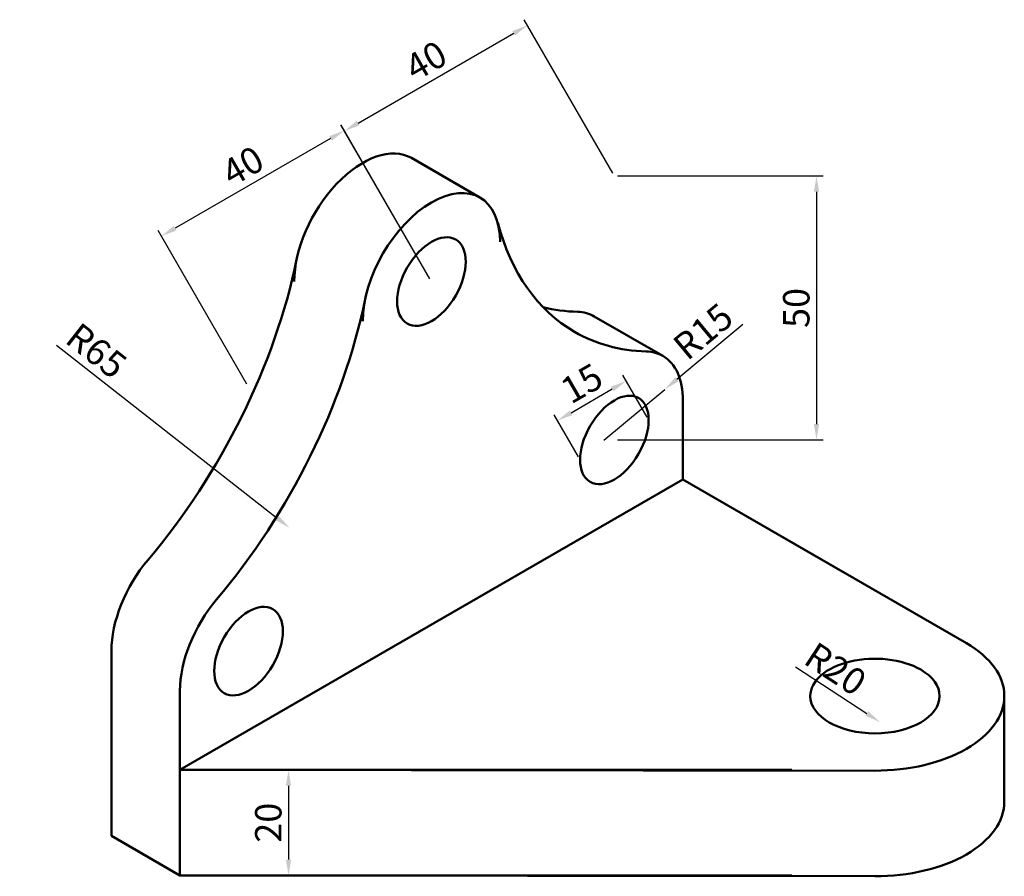
# Model space of a CAD drawing. Units: millimetres. Extents: x 6 to 193, y 3 to 166.
import ezdxf

# ---------------------------------------------------------------- set-up
doc = ezdxf.new("R2010")
doc.units = ezdxf.units.MM
doc.layers.add('M-DIMS', color=2, linetype='Continuous', lineweight=25)
doc.layers.add('M-OUTL', color=7, linetype='Continuous', lineweight=50)
doc.styles.get("Standard").update_dxf_attribs({"font": 'arial.ttf'})
doc.dimstyles.new('ISO-25', dxfattribs={"dimtxt": 5, "dimasz": 3, "dimexe": 1.25, "dimexo": 0.625, "dimtad": 1, "dimtxsty": 'Standard', "dimcen": 2.5, "dimadec": 0, "dimazin": 0, "dimtfac": 1, "dimtmove": 0, "dimatfit": 3, "dimfxl": 1, "dimarcsym": 0})

# ---------------------------------------------------------------- blocks, each defined once
blk = doc.blocks.new('*D1')
at = {"layer": 'Defpoints', "color": 0, "transparency": 16777216}
for p in [(118.67, 136.1), (118.67, 86.1), (156.96, 86.1)]:
    blk.add_point(p, dxfattribs=at)
at = {"layer": 'M-DIMS', "color": 0, "lineweight": -2, "transparency": 16777216}
for p, q in [((119.3, 136.1), (158.21, 136.1)), ((156.96, 133.1), (156.96, 89.1)), ((119.3, 86.1), (158.21, 86.1))]:
    blk.add_line(p, q, dxfattribs=at)
at = {"layer": 'M-DIMS', "color": 0, "transparency": 16777216}
for points in [[(156.46, 133.1), (157.46, 133.1), (156.96, 136.1)], [(156.46, 89.1), (157.46, 89.1), (156.96, 86.1)]]:
    blk.add_solid(points, dxfattribs=at)
at = {"layer": 'M-DIMS', "color": 0, "transparency": 16777216, "insert": (153.78, 111.1), "char_height": 5, "attachment_point": 5, "rotation": 90}
blk.add_mtext('50', dxfattribs=at)
blk = doc.blocks.new('*D2')
at = {"layer": 'Defpoints', "color": 0, "transparency": 16777216}
for p in [(102.21, 164.62), (118.67, 136.1), (84.03, 116.1)]:
    blk.add_point(p, dxfattribs=at)
at = {"layer": 'M-DIMS', "color": 0, "lineweight": -2, "transparency": 16777216}
for p, q in [((118.36, 136.64), (101.58, 165.7)), ((70.16, 146.12), (99.61, 163.12)), ((83.72, 116.64), (66.94, 145.7))]:
    blk.add_line(p, q, dxfattribs=at)
at = {"layer": 'M-DIMS', "color": 0, "transparency": 16777216}
for points in [[(99.36, 163.55), (99.86, 162.69), (102.21, 164.62)], [(69.91, 146.55), (70.41, 145.69), (67.56, 144.62)]]:
    blk.add_solid(points, dxfattribs=at)
at = {"layer": 'M-DIMS', "color": 0, "transparency": 16777216, "insert": (83.3, 157.37), "char_height": 5, "attachment_point": 5, "rotation": 30}
blk.add_mtext('40', dxfattribs=at)
blk = doc.blocks.new('*D3')
at = {"layer": 'Defpoints', "color": 0, "transparency": 16777216}
for p in [(32.88, 124.7), (84.03, 116.1), (49.39, 96.1)]:
    blk.add_point(p, dxfattribs=at)
at = {"layer": 'M-DIMS', "color": 0, "lineweight": -2, "transparency": 16777216}
for p, q in [((83.72, 116.64), (66.89, 145.78)), ((64.92, 143.2), (35.48, 126.2)), ((49.08, 96.64), (32.25, 125.78))]:
    blk.add_line(p, q, dxfattribs=at)
at = {"layer": 'M-DIMS', "color": 0, "transparency": 16777216}
for points in [[(64.67, 143.63), (65.17, 142.76), (67.52, 144.7)], [(35.23, 126.63), (35.73, 125.76), (32.88, 124.7)]]:
    blk.add_solid(points, dxfattribs=at)
at = {"layer": 'M-DIMS', "color": 0, "transparency": 16777216, "insert": (48.61, 137.45), "char_height": 5, "attachment_point": 5, "rotation": 30}
blk.add_mtext('40', dxfattribs=at)
blk = doc.blocks.new('*D4')
at = {"layer": 'Defpoints', "color": 0, "transparency": 16777216}
for p in [(36.4, 23.6), (36.4, 3.6), (56.96, 3.6)]:
    blk.add_point(p, dxfattribs=at)
at = {"layer": 'M-DIMS', "color": 0, "lineweight": -2, "transparency": 16777216}
for p, q in [((37.03, 23.6), (58.21, 23.6)), ((56.96, 20.6), (56.96, 6.6)), ((37.03, 3.6), (58.21, 3.6))]:
    blk.add_line(p, q, dxfattribs=at)
at = {"layer": 'M-DIMS', "color": 0, "transparency": 16777216}
for points in [[(56.46, 20.6), (57.46, 20.6), (56.96, 23.6)], [(56.46, 6.6), (57.46, 6.6), (56.96, 3.6)]]:
    blk.add_solid(points, dxfattribs=at)
at = {"layer": 'M-DIMS', "color": 0, "transparency": 16777216, "insert": (53.78, 13.6), "char_height": 5, "attachment_point": 5, "rotation": 90}
blk.add_mtext('20', dxfattribs=at)
blk = doc.blocks.new('*D5')
at = {"layer": 'Defpoints', "color": 0, "transparency": 16777216}
for p in [(152.28, 43.6), (169.01, 32.63)]:
    blk.add_point(p, dxfattribs=at)
at = {"layer": 'M-DIMS', "color": 0, "lineweight": -2, "transparency": 16777216}
blk.add_line((152.97, 43.15), (166.5, 34.28), dxfattribs=at)
at = {"layer": 'M-DIMS', "color": 0, "transparency": 16777216}
blk.add_solid([(166.78, 34.7), (166.23, 33.86), (169.01, 32.63)], dxfattribs=at)
at = {"layer": 'M-DIMS', "color": 0, "transparency": 16777216, "insert": (160.22, 42.19), "char_height": 5, "attachment_point": 5, "rotation": 326.7605}
blk.add_mtext('R20', dxfattribs=at)
blk = doc.blocks.new('*D6')
at = {"layer": 'Defpoints', "color": 0, "transparency": 16777216}
for p in [(6.05, 109.54), (57.2, 69.43)]:
    blk.add_point(p, dxfattribs=at)
at = {"layer": 'M-DIMS', "color": 0, "lineweight": -2, "transparency": 16777216}
blk.add_line((13.02, 104.07), (54.84, 71.28), dxfattribs=at)
at = {"layer": 'M-DIMS', "color": 0, "transparency": 16777216}
blk.add_solid([(55.15, 71.67), (54.53, 70.88), (57.2, 69.43)], dxfattribs=at)
at = {"layer": 'M-DIMS', "color": 0, "transparency": 16777216, "insert": (20.19, 102.49), "char_height": 5, "attachment_point": 5, "rotation": 321.8978}
blk.add_mtext('R65', dxfattribs=at)
blk = doc.blocks.new('*D7')
at = {"layer": 'Defpoints', "color": 0, "transparency": 16777216}
for p in [(128.21, 95.66), (116.66, 86.08)]:
    blk.add_point(p, dxfattribs=at)
at = {"layer": 'M-DIMS', "color": 0, "lineweight": -2, "transparency": 16777216}
for p, q in [((143.01, 107.94), (130.52, 97.57)), ((116.66, 86.08), (128.21, 95.66))]:
    blk.add_line(p, q, dxfattribs=at)
at = {"layer": 'M-DIMS', "color": 0, "transparency": 16777216}
blk.add_solid([(130.2, 97.96), (130.83, 97.19), (128.21, 95.66)], dxfattribs=at)
at = {"layer": 'M-DIMS', "color": 0, "transparency": 16777216, "insert": (135.89, 106.16), "char_height": 5, "attachment_point": 5, "rotation": 39.6852}
blk.add_mtext('R15', dxfattribs=at)
blk = doc.blocks.new('*D8')
at = {"layer": 'Defpoints', "color": 0, "transparency": 16777216}
for p in [(120.89, 97.25), (125.17, 89.85), (112.18, 82.35)]:
    blk.add_point(p, dxfattribs=at)
at = {"layer": 'M-DIMS', "color": 0, "lineweight": -2, "transparency": 16777216}
for p, q in [((124.86, 90.39), (120.27, 98.34)), ((110.5, 91.25), (118.29, 95.75)), ((111.86, 82.89), (107.28, 90.84))]:
    blk.add_line(p, q, dxfattribs=at)
at = {"layer": 'M-DIMS', "color": 0, "transparency": 16777216}
for points in [[(118.04, 96.19), (118.54, 95.32), (120.89, 97.25)], [(110.25, 91.69), (110.75, 90.82), (107.9, 89.75)]]:
    blk.add_solid(points, dxfattribs=at)
at = {"layer": 'M-DIMS', "color": 0, "transparency": 16777216, "insert": (112.81, 96.26), "char_height": 5, "attachment_point": 5, "rotation": 30}
blk.add_mtext('15', dxfattribs=at)

msp = doc.modelspace()

# ---------------------------------------------------------------- linework, layer by layer
at = {"layer": 'M-OUTL'}
for p, q in [((80.227, 139.506), (93.217, 132.006)), ((114.868, 109.506), (127.858, 102.006)), ((131.663, 78.596), (131.663, 93.596)), ((131.663, 86.08), (131.663, 78.596)), ((36.4, 23.596), (131.663, 78.596)), ((131.663, 78.596), (162.285, 60.916)), ((185.357, 47.596), (131.663, 78.596)), ((23.41, 46.096), (23.41, 31.096)), ((36.4, 38.596), (36.4, 23.596)), ((192.531, 37.596), (192.531, 17.596)), ((23.41, 31.096), (23.41, 11.096)), ((36.4, 23.596), (36.4, 3.596)), ((36.4, 23.596), (152.285, 23.596)), ((36.4, 23.596), (167.99, 23.454)), ((36.4, 3.596), (23.41, 11.096)), ((36.4, 3.596), (152.285, 3.596)), ((36.4, 3.596), (167.99, 3.454))]:
    msp.add_line(p, q, dxfattribs=at)
for centre, major_axis, start_param, end_param in [((71.041, 123.596), (-9.186, -15.91), 3.1415927, 5.4977871), ((84.032, 116.096), (-9.186, -15.91), 2.3561945, 5.4977871), ((150.931, 175.519), (39.804, 68.943), 2.6192054, 3.1415927), ((4.142, 105.77), (39.804, 68.943), 4.4113162, 5.2347762), ((17.132, 98.27), (39.804, 68.943), 4.4113162, 5.2347762), ((137.941, 183.019), (39.804, 68.943), 3.3055042, 3.4426655), ((105.682, 93.596), (-9.186, -15.91), 3.1415927, 3.4426655), ((150.931, 175.519), (39.804, 68.943), 3.1415927, 3.4426655), ((118.673, 86.096), (-9.186, -15.91), 3.1415927, 3.4426655), ((118.673, 86.096), (-9.186, -15.91), 2.3561944, 3.1415927), ((36.4, 53.596), (-9.186, -15.91), 4.4113162, 5.4977873), ((49.391, 46.096), (-9.186, -15.91), 4.4113162, 5.4977873), ((168.036, 37.596), (24.495, 0), 0, 0.7853996), ((168.036, 37.596), (12.247, 0), 0.7853982, 3.1415927), ((168.036, 37.596), (12.247, 0), 0, 0.7853982), ((168.036, 37.596), (12.247, 0), 3.1415927, 6.2831853), ((168.036, 37.596), (24.495, 0), 4.7105162, 6.2831853), ((168.036, 17.596), (24.495, 0), 4.7105162, 6.2831853)]:
    msp.add_ellipse(centre, major_axis=major_axis, ratio=0.5773503, start_param=start_param, end_param=end_param, dxfattribs=at)
for centre in [(84.032, 116.096), (118.673, 86.096), (49.391, 46.096)]:
    msp.add_ellipse(centre, major_axis=(-4.593, -7.955), ratio=0.5773503, dxfattribs=at)

# ---------------------------------------------------------------- dimensions: what is measured, and where the dimension line sits
at = {"layer": 'M-DIMS'}
for p1, p2, distance, picture, middle in [((84.032, 116.096), (118.673, 136.096), 32.935, '*D2', (83.296, 157.37)), ((84.032, 116.096), (49.391, 96.096), -33.026, '*D3', (48.609, 137.449)), ((112.177, 82.346), (125.168, 89.846), 8.554, '*D8', (112.807, 96.256))]:
    dim = msp.add_aligned_dim(p1=p1, p2=p2, distance=distance, dimstyle='ISO-25', override={"dimclrd": 0, "dimclre": 0, "dimclrt": 0}, dxfattribs=at)
    dim.commit()
    dim.dimension.update_dxf_attribs({"geometry": picture, "text_midpoint": middle})
for base, p1, p2, picture, middle in [((156.961, 86.096), (118.673, 136.096), (118.673, 86.096), '*D1', (153.783, 111.096)), ((56.96, 3.596), (36.4, 23.596), (36.4, 3.596), '*D4', (53.783, 13.596))]:
    dim = msp.add_linear_dim(base=base, p1=p1, p2=p2, angle=90, dimstyle='ISO-25', override={"dimclrd": 0, "dimclre": 0, "dimclrt": 0}, dxfattribs=at)
    dim.commit()
    dim.dimension.update_dxf_attribs({"geometry": picture, "text_midpoint": middle})
dim = msp.add_radius_dim(center=(116.663, 86.08), mpoint=(128.206, 95.658), dimstyle='ISO-25', override={"dimclrd": 0, "dimclre": 0, "dimclrt": 0}, dxfattribs=at)
dim.commit()
dim.dimension.update_dxf_attribs({"geometry": '*D7', "text_midpoint": (135.887, 106.161)})
for center, mpoint, picture, middle in [((6.048, 109.536), (57.197, 69.426), '*D6', (18.227, 99.985)), ((152.285, 43.596), (169.012, 32.633), '*D5', (158.482, 39.534))]:
    dim = msp.add_radius_dim(center=center, mpoint=mpoint, dimstyle='ISO-25', override={"dimclrd": 0, "dimclre": 0, "dimclrt": 0}, dxfattribs=at)
    dim.commit()
    dim.dimension.update_dxf_attribs({"geometry": picture, "text_midpoint": middle, "dimtype": 164})

doc.saveas('drawing.dxf')
